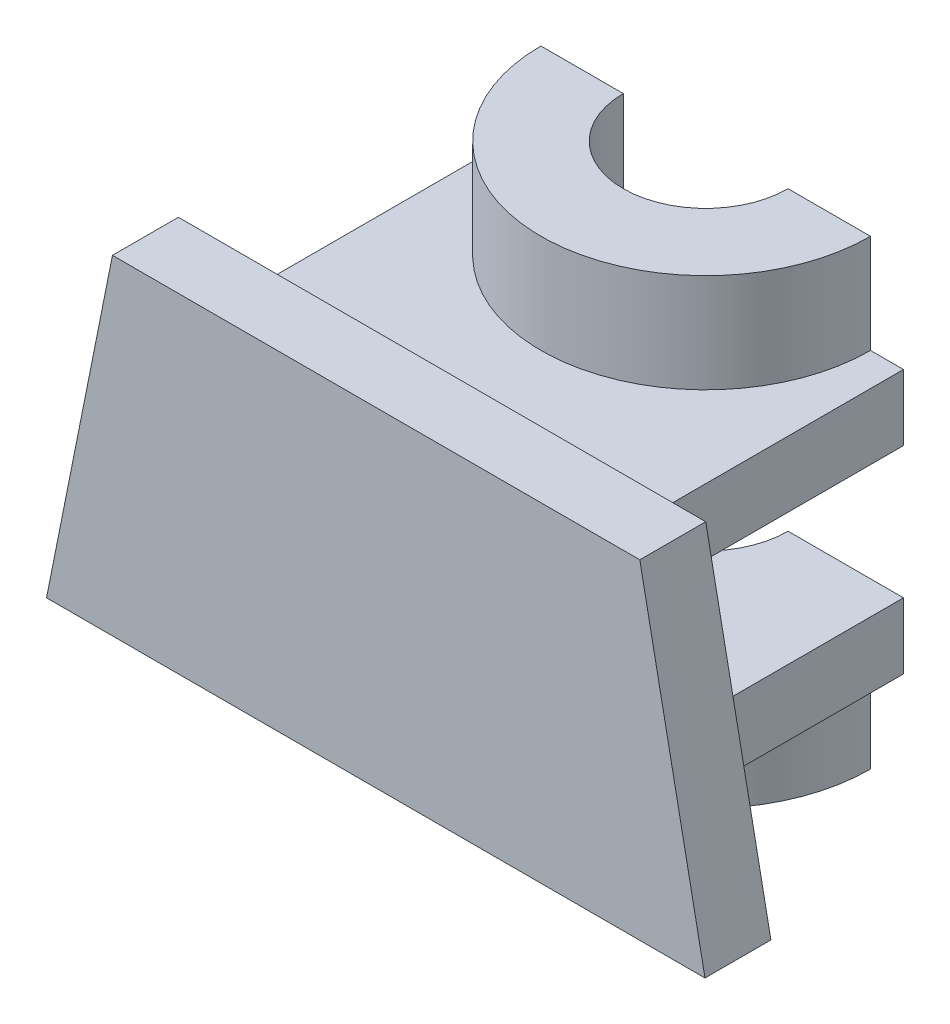
ISO-10303-21;
HEADER;
FILE_DESCRIPTION(('STEP AP214'),'2;1');
FILE_NAME('part.step','',(''),(''),'','','');
FILE_SCHEMA(('AUTOMOTIVE_DESIGN { 1 0 10303 214 1 1 1 1 }'));
ENDSEC;
DATA;
#1=APPLICATION_CONTEXT('core data for automotive mechanical design processes');
#2=APPLICATION_PROTOCOL_DEFINITION('international standard','automotive_design',2000,#1);
#3=PRODUCT_CONTEXT('',#1,'mechanical');
#4=PRODUCT('Part','Part','',(#3));
#5=PRODUCT_RELATED_PRODUCT_CATEGORY('part','',(#4));
#6=PRODUCT_DEFINITION_FORMATION('','',#4);
#7=PRODUCT_DEFINITION_CONTEXT('part definition',#1,'design');
#8=PRODUCT_DEFINITION('design','',#6,#7);
#9=PRODUCT_DEFINITION_SHAPE('','',#8);
#10=(LENGTH_UNIT() NAMED_UNIT(*) SI_UNIT(.MILLI.,.METRE.));
#11=(NAMED_UNIT(*) PLANE_ANGLE_UNIT() SI_UNIT($,.RADIAN.));
#12=(NAMED_UNIT(*) SI_UNIT($,.STERADIAN.) SOLID_ANGLE_UNIT());
#13=UNCERTAINTY_MEASURE_WITH_UNIT(LENGTH_MEASURE(1.E-05),#10,'distance_accuracy_value','');
#14=(GEOMETRIC_REPRESENTATION_CONTEXT(3) GLOBAL_UNCERTAINTY_ASSIGNED_CONTEXT((#13)) GLOBAL_UNIT_ASSIGNED_CONTEXT((#10,
#11,#12)) REPRESENTATION_CONTEXT('',''));
#15=CARTESIAN_POINT('',(0.,0.,0.));
#16=DIRECTION('',(0.,0.,1.));
#17=DIRECTION('',(1.,0.,0.));
#18=AXIS2_PLACEMENT_3D('',#15,#16,#17);
#19=CARTESIAN_POINT('',(0.,45.,0.));
#20=DIRECTION('',(0.,-1.,0.));
#21=DIRECTION('',(0.,0.,-1.));
#22=AXIS2_PLACEMENT_3D('',#19,#20,#21);
#23=PLANE('',#22);
#24=CARTESIAN_POINT('',(50.,45.,-40.));
#25=DIRECTION('',(0.,1.,0.));
#26=DIRECTION('',(0.,0.,1.));
#27=AXIS2_PLACEMENT_3D('',#24,#25,#26);
#28=CIRCLE('',#27,25.);
#29=CARTESIAN_POINT('',(25.,45.,-40.));
#30=VERTEX_POINT('',#29);
#31=CARTESIAN_POINT('',(75.,45.,-40.));
#32=VERTEX_POINT('',#31);
#33=EDGE_CURVE('E293',#30,#32,#28,.T.);
#34=ORIENTED_EDGE('',*,*,#33,.F.);
#35=DIRECTION('',(-1.,0.,0.));
#36=VECTOR('',#35,1.);
#37=CARTESIAN_POINT('',(20.,45.,-40.));
#38=LINE('',#37,#36);
#39=CARTESIAN_POINT('',(20.,45.,-40.));
#40=VERTEX_POINT('',#39);
#41=EDGE_CURVE('E221',#30,#40,#38,.T.);
#42=ORIENTED_EDGE('',*,*,#41,.T.);
#43=DIRECTION('',(0.,0.,1.));
#44=VECTOR('',#43,1.);
#45=CARTESIAN_POINT('',(20.,45.,0.));
#46=LINE('',#45,#44);
#47=CARTESIAN_POINT('',(20.,45.,0.));
#48=VERTEX_POINT('',#47);
#49=EDGE_CURVE('E216',#40,#48,#46,.T.);
#50=ORIENTED_EDGE('',*,*,#49,.T.);
#51=DIRECTION('',(1.,0.,0.));
#52=VECTOR('',#51,1.);
#53=CARTESIAN_POINT('',(50.,45.,0.));
#54=LINE('',#53,#52);
#55=CARTESIAN_POINT('',(80.,45.,0.));
#56=VERTEX_POINT('',#55);
#57=EDGE_CURVE('E213',#48,#56,#54,.T.);
#58=ORIENTED_EDGE('',*,*,#57,.T.);
#59=DIRECTION('',(0.,0.,-1.));
#60=VECTOR('',#59,1.);
#61=CARTESIAN_POINT('',(80.,45.,-40.));
#62=LINE('',#61,#60);
#63=CARTESIAN_POINT('',(80.,45.,-40.));
#64=VERTEX_POINT('',#63);
#65=EDGE_CURVE('E228',#56,#64,#62,.T.);
#66=ORIENTED_EDGE('',*,*,#65,.T.);
#67=EDGE_CURVE('E225',#64,#32,#38,.T.);
#68=ORIENTED_EDGE('',*,*,#67,.T.);
#69=EDGE_LOOP('',(#34,#42,#50,#58,#66,#68));
#70=FACE_BOUND('',#69,.T.);
#71=ADVANCED_FACE('F39',(#70),#23,.F.);
#72=CARTESIAN_POINT('',(20.,35.,-40.));
#73=DIRECTION('',(0.,0.,-1.));
#74=DIRECTION('',(-1.,0.,0.));
#75=AXIS2_PLACEMENT_3D('',#72,#73,#74);
#76=PLANE('',#75);
#77=DIRECTION('',(0.,1.,0.));
#78=VECTOR('',#77,1.);
#79=CARTESIAN_POINT('',(37.5,0.,-40.));
#80=LINE('',#79,#78);
#81=CARTESIAN_POINT('',(37.5,35.,-40.));
#82=VERTEX_POINT('',#81);
#83=CARTESIAN_POINT('',(37.5,60.,-40.));
#84=VERTEX_POINT('',#83);
#85=EDGE_CURVE('E264',#82,#84,#80,.T.);
#86=ORIENTED_EDGE('',*,*,#85,.F.);
#87=DIRECTION('',(-1.,0.,0.));
#88=VECTOR('',#87,1.);
#89=CARTESIAN_POINT('',(20.,35.,-40.));
#90=LINE('',#89,#88);
#91=CARTESIAN_POINT('',(20.,35.,-40.));
#92=VERTEX_POINT('',#91);
#93=EDGE_CURVE('E232',#82,#92,#90,.T.);
#94=ORIENTED_EDGE('',*,*,#93,.T.);
#95=DIRECTION('',(0.,1.,0.));
#96=VECTOR('',#95,1.);
#97=CARTESIAN_POINT('',(20.,35.,-40.));
#98=LINE('',#97,#96);
#99=EDGE_CURVE('E208',#92,#40,#98,.T.);
#100=ORIENTED_EDGE('',*,*,#99,.T.);
#101=ORIENTED_EDGE('',*,*,#41,.F.);
#102=DIRECTION('',(0.,-1.,0.));
#103=VECTOR('',#102,1.);
#104=CARTESIAN_POINT('',(25.,60.,-40.));
#105=LINE('',#104,#103);
#106=CARTESIAN_POINT('',(25.,60.,-40.));
#107=VERTEX_POINT('',#106);
#108=EDGE_CURVE('E288',#107,#30,#105,.T.);
#109=ORIENTED_EDGE('',*,*,#108,.F.);
#110=DIRECTION('',(-1.,0.,0.));
#111=VECTOR('',#110,1.);
#112=CARTESIAN_POINT('',(25.,60.,-40.));
#113=LINE('',#112,#111);
#114=EDGE_CURVE('E286',#84,#107,#113,.T.);
#115=ORIENTED_EDGE('',*,*,#114,.F.);
#116=EDGE_LOOP('',(#86,#94,#100,#101,#109,#115));
#117=FACE_BOUND('',#116,.T.);
#118=ADVANCED_FACE('F345',(#117),#76,.T.);
#119=CARTESIAN_POINT('',(20.,15.,-40.));
#120=DIRECTION('',(0.,0.,1.));
#121=DIRECTION('',(1.,0.,0.));
#122=AXIS2_PLACEMENT_3D('',#119,#120,#121);
#123=PLANE('',#122);
#124=DIRECTION('',(-1.,0.,0.));
#125=VECTOR('',#124,1.);
#126=CARTESIAN_POINT('',(20.,5.,-40.));
#127=LINE('',#126,#125);
#128=CARTESIAN_POINT('',(80.,5.,-40.));
#129=VERTEX_POINT('',#128);
#130=CARTESIAN_POINT('',(75.,5.,-40.));
#131=VERTEX_POINT('',#130);
#132=EDGE_CURVE('E251',#129,#131,#127,.T.);
#133=ORIENTED_EDGE('',*,*,#132,.T.);
#134=DIRECTION('',(0.,1.,0.));
#135=VECTOR('',#134,1.);
#136=CARTESIAN_POINT('',(75.,-9.99999999999999,-40.));
#137=LINE('',#136,#135);
#138=CARTESIAN_POINT('',(75.,-9.99999999999999,-40.));
#139=VERTEX_POINT('',#138);
#140=EDGE_CURVE('E310',#139,#131,#137,.T.);
#141=ORIENTED_EDGE('',*,*,#140,.F.);
#142=DIRECTION('',(-1.,0.,0.));
#143=VECTOR('',#142,1.);
#144=CARTESIAN_POINT('',(62.5,-9.99999999999999,-40.));
#145=LINE('',#144,#143);
#146=CARTESIAN_POINT('',(62.5,-9.99999999999999,-40.));
#147=VERTEX_POINT('',#146);
#148=EDGE_CURVE('E309',#139,#147,#145,.T.);
#149=ORIENTED_EDGE('',*,*,#148,.T.);
#150=DIRECTION('',(0.,1.,0.));
#151=VECTOR('',#150,1.);
#152=CARTESIAN_POINT('',(62.5,0.,-40.));
#153=LINE('',#152,#151);
#154=CARTESIAN_POINT('',(62.5,15.,-40.));
#155=VERTEX_POINT('',#154);
#156=EDGE_CURVE('E282',#147,#155,#153,.T.);
#157=ORIENTED_EDGE('',*,*,#156,.T.);
#158=DIRECTION('',(-1.,0.,0.));
#159=VECTOR('',#158,1.);
#160=CARTESIAN_POINT('',(20.,15.,-40.));
#161=LINE('',#160,#159);
#162=CARTESIAN_POINT('',(80.,15.,-40.));
#163=VERTEX_POINT('',#162);
#164=EDGE_CURVE('E263',#163,#155,#161,.T.);
#165=ORIENTED_EDGE('',*,*,#164,.F.);
#166=DIRECTION('',(0.,-1.,0.));
#167=VECTOR('',#166,1.);
#168=CARTESIAN_POINT('',(80.,15.,-40.));
#169=LINE('',#168,#167);
#170=EDGE_CURVE('E246',#163,#129,#169,.T.);
#171=ORIENTED_EDGE('',*,*,#170,.T.);
#172=EDGE_LOOP('',(#133,#141,#149,#157,#165,#171));
#173=FACE_BOUND('',#172,.T.);
#174=ADVANCED_FACE('F346',(#173),#123,.F.);
#175=CARTESIAN_POINT('',(0.,0.,10.));
#176=DIRECTION('',(0.,1.,0.));
#177=DIRECTION('',(0.,0.,1.));
#178=AXIS2_PLACEMENT_3D('',#175,#176,#177);
#179=PLANE('',#178);
#180=DIRECTION('',(1.,0.,0.));
#181=VECTOR('',#180,1.);
#182=CARTESIAN_POINT('',(0.,0.,0.));
#183=LINE('',#182,#181);
#184=CARTESIAN_POINT('',(0.,0.,0.));
#185=VERTEX_POINT('',#184);
#186=CARTESIAN_POINT('',(99.8906286080262,0.,0.));
#187=VERTEX_POINT('',#186);
#188=EDGE_CURVE('E195',#185,#187,#183,.T.);
#189=ORIENTED_EDGE('',*,*,#188,.T.);
#190=DIRECTION('',(0.,0.,1.));
#191=VECTOR('',#190,1.);
#192=CARTESIAN_POINT('',(99.8906286080262,0.,10.));
#193=LINE('',#192,#191);
#194=CARTESIAN_POINT('',(99.8906286080262,0.,10.));
#195=VERTEX_POINT('',#194);
#196=EDGE_CURVE('E53',#187,#195,#193,.T.);
#197=ORIENTED_EDGE('',*,*,#196,.T.);
#198=DIRECTION('',(1.,0.,0.));
#199=VECTOR('',#198,1.);
#200=CARTESIAN_POINT('',(0.,0.,10.));
#201=LINE('',#200,#199);
#202=CARTESIAN_POINT('',(0.,0.,10.));
#203=VERTEX_POINT('',#202);
#204=EDGE_CURVE('E192',#203,#195,#201,.T.);
#205=ORIENTED_EDGE('',*,*,#204,.F.);
#206=DIRECTION('',(0.,0.,-1.));
#207=VECTOR('',#206,1.);
#208=CARTESIAN_POINT('',(0.,0.,10.));
#209=LINE('',#208,#207);
#210=EDGE_CURVE('E50',#203,#185,#209,.T.);
#211=ORIENTED_EDGE('',*,*,#210,.T.);
#212=EDGE_LOOP('',(#189,#197,#205,#211));
#213=FACE_BOUND('',#212,.T.);
#214=ADVANCED_FACE('F41',(#213),#179,.F.);
#215=CARTESIAN_POINT('',(100.,50.,10.));
#216=DIRECTION('',(0.,-1.,0.));
#217=DIRECTION('',(0.,0.,-1.));
#218=AXIS2_PLACEMENT_3D('',#215,#216,#217);
#219=PLANE('',#218);
#220=DIRECTION('',(-1.,0.,0.));
#221=VECTOR('',#220,1.);
#222=CARTESIAN_POINT('',(100.,50.,10.));
#223=LINE('',#222,#221);
#224=CARTESIAN_POINT('',(90.,50.,10.));
#225=VERTEX_POINT('',#224);
#226=CARTESIAN_POINT('',(9.99999999999999,50.,10.));
#227=VERTEX_POINT('',#226);
#228=EDGE_CURVE('E187',#225,#227,#223,.T.);
#229=ORIENTED_EDGE('',*,*,#228,.F.);
#230=DIRECTION('',(0.,0.,-1.));
#231=VECTOR('',#230,1.);
#232=CARTESIAN_POINT('',(90.,50.,15.));
#233=LINE('',#232,#231);
#234=CARTESIAN_POINT('',(90.,50.,0.));
#235=VERTEX_POINT('',#234);
#236=EDGE_CURVE('E172',#225,#235,#233,.T.);
#237=ORIENTED_EDGE('',*,*,#236,.T.);
#238=DIRECTION('',(-1.,0.,0.));
#239=VECTOR('',#238,1.);
#240=CARTESIAN_POINT('',(100.,50.,0.));
#241=LINE('',#240,#239);
#242=CARTESIAN_POINT('',(9.99999999999999,50.,0.));
#243=VERTEX_POINT('',#242);
#244=EDGE_CURVE('E183',#235,#243,#241,.T.);
#245=ORIENTED_EDGE('',*,*,#244,.T.);
#246=DIRECTION('',(0.,0.,-1.));
#247=VECTOR('',#246,1.);
#248=CARTESIAN_POINT('',(9.99999999999999,50.,15.));
#249=LINE('',#248,#247);
#250=EDGE_CURVE('E62',#227,#243,#249,.T.);
#251=ORIENTED_EDGE('',*,*,#250,.F.);
#252=EDGE_LOOP('',(#229,#237,#245,#251));
#253=FACE_BOUND('',#252,.T.);
#254=ADVANCED_FACE('F182',(#253),#219,.F.);
#255=CARTESIAN_POINT('',(0.,0.,10.));
#256=DIRECTION('',(0.,0.,1.));
#257=DIRECTION('',(1.,0.,0.));
#258=AXIS2_PLACEMENT_3D('',#255,#256,#257);
#259=PLANE('',#258);
#260=DIRECTION('',(0.194052386180956,-0.980991167859057,0.));
#261=VECTOR('',#260,1.);
#262=CARTESIAN_POINT('',(96.1291142748476,19.0155473542205,10.));
#263=LINE('',#262,#261);
#264=EDGE_CURVE('E323',#225,#195,#263,.T.);
#265=ORIENTED_EDGE('',*,*,#264,.F.);
#266=ORIENTED_EDGE('',*,*,#228,.T.);
#267=DIRECTION('',(0.196116135138184,0.98058067569092,0.));
#268=VECTOR('',#267,1.);
#269=CARTESIAN_POINT('',(0.,0.,10.));
#270=LINE('',#269,#268);
#271=EDGE_CURVE('E190',#203,#227,#270,.T.);
#272=ORIENTED_EDGE('',*,*,#271,.F.);
#273=ORIENTED_EDGE('',*,*,#204,.T.);
#274=EDGE_LOOP('',(#265,#266,#272,#273));
#275=FACE_BOUND('',#274,.T.);
#276=ADVANCED_FACE('F328',(#275),#259,.T.);
#277=CARTESIAN_POINT('',(0.,0.,0.));
#278=DIRECTION('',(0.,0.,1.));
#279=DIRECTION('',(1.,0.,0.));
#280=AXIS2_PLACEMENT_3D('',#277,#278,#279);
#281=PLANE('',#280);
#282=DIRECTION('',(0.,-1.,0.));
#283=VECTOR('',#282,1.);
#284=CARTESIAN_POINT('',(80.,15.,0.));
#285=LINE('',#284,#283);
#286=CARTESIAN_POINT('',(80.,15.,0.));
#287=VERTEX_POINT('',#286);
#288=CARTESIAN_POINT('',(80.,5.,0.));
#289=VERTEX_POINT('',#288);
#290=EDGE_CURVE('E230',#287,#289,#285,.T.);
#291=ORIENTED_EDGE('',*,*,#290,.F.);
#292=DIRECTION('',(1.,0.,0.));
#293=VECTOR('',#292,1.);
#294=CARTESIAN_POINT('',(80.,15.,0.));
#295=LINE('',#294,#293);
#296=CARTESIAN_POINT('',(20.,15.,0.));
#297=VERTEX_POINT('',#296);
#298=EDGE_CURVE('E254',#297,#287,#295,.T.);
#299=ORIENTED_EDGE('',*,*,#298,.F.);
#300=DIRECTION('',(0.,-1.,0.));
#301=VECTOR('',#300,1.);
#302=CARTESIAN_POINT('',(20.,15.,0.));
#303=LINE('',#302,#301);
#304=CARTESIAN_POINT('',(20.,5.,0.));
#305=VERTEX_POINT('',#304);
#306=EDGE_CURVE('E239',#297,#305,#303,.T.);
#307=ORIENTED_EDGE('',*,*,#306,.T.);
#308=DIRECTION('',(1.,0.,0.));
#309=VECTOR('',#308,1.);
#310=CARTESIAN_POINT('',(50.,5.,0.));
#311=LINE('',#310,#309);
#312=EDGE_CURVE('E262',#305,#289,#311,.T.);
#313=ORIENTED_EDGE('',*,*,#312,.T.);
#314=EDGE_LOOP('',(#291,#299,#307,#313));
#315=FACE_BOUND('',#314,.T.);
#316=DIRECTION('',(0.,1.,0.));
#317=VECTOR('',#316,1.);
#318=CARTESIAN_POINT('',(20.,35.,0.));
#319=LINE('',#318,#317);
#320=CARTESIAN_POINT('',(20.,35.,0.));
#321=VERTEX_POINT('',#320);
#322=EDGE_CURVE('E197',#321,#48,#319,.T.);
#323=ORIENTED_EDGE('',*,*,#322,.F.);
#324=DIRECTION('',(1.,0.,0.));
#325=VECTOR('',#324,1.);
#326=CARTESIAN_POINT('',(80.,35.,0.));
#327=LINE('',#326,#325);
#328=CARTESIAN_POINT('',(80.,35.,0.));
#329=VERTEX_POINT('',#328);
#330=EDGE_CURVE('E219',#321,#329,#327,.T.);
#331=ORIENTED_EDGE('',*,*,#330,.T.);
#332=DIRECTION('',(0.,1.,0.));
#333=VECTOR('',#332,1.);
#334=CARTESIAN_POINT('',(80.,35.,0.));
#335=LINE('',#334,#333);
#336=EDGE_CURVE('E201',#329,#56,#335,.T.);
#337=ORIENTED_EDGE('',*,*,#336,.T.);
#338=ORIENTED_EDGE('',*,*,#57,.F.);
#339=EDGE_LOOP('',(#323,#331,#337,#338));
#340=FACE_BOUND('',#339,.T.);
#341=ORIENTED_EDGE('',*,*,#244,.F.);
#342=DIRECTION('',(0.194052386180956,-0.980991167859057,0.));
#343=VECTOR('',#342,1.);
#344=CARTESIAN_POINT('',(96.1291142748476,19.0155473542205,0.));
#345=LINE('',#344,#343);
#346=EDGE_CURVE('E11',#235,#187,#345,.T.);
#347=ORIENTED_EDGE('',*,*,#346,.T.);
#348=ORIENTED_EDGE('',*,*,#188,.F.);
#349=DIRECTION('',(-0.196116135138184,-0.98058067569092,0.));
#350=VECTOR('',#349,1.);
#351=CARTESIAN_POINT('',(9.99999999999999,50.,0.));
#352=LINE('',#351,#350);
#353=EDGE_CURVE('E188',#243,#185,#352,.T.);
#354=ORIENTED_EDGE('',*,*,#353,.F.);
#355=EDGE_LOOP('',(#341,#347,#348,#354));
#356=FACE_BOUND('',#355,.T.);
#357=ADVANCED_FACE('F186',(#315,#340,#356),#281,.F.);
#358=CARTESIAN_POINT('',(20.,35.,0.));
#359=DIRECTION('',(-1.,0.,0.));
#360=DIRECTION('',(0.,0.,1.));
#361=AXIS2_PLACEMENT_3D('',#358,#359,#360);
#362=PLANE('',#361);
#363=ORIENTED_EDGE('',*,*,#49,.F.);
#364=ORIENTED_EDGE('',*,*,#99,.F.);
#365=DIRECTION('',(0.,0.,1.));
#366=VECTOR('',#365,1.);
#367=CARTESIAN_POINT('',(20.,35.,0.));
#368=LINE('',#367,#366);
#369=EDGE_CURVE('E206',#92,#321,#368,.T.);
#370=ORIENTED_EDGE('',*,*,#369,.T.);
#371=ORIENTED_EDGE('',*,*,#322,.T.);
#372=EDGE_LOOP('',(#363,#364,#370,#371));
#373=FACE_BOUND('',#372,.T.);
#374=ADVANCED_FACE('F340',(#373),#362,.T.);
#375=DIRECTION('',(0.,1.,0.));
#376=VECTOR('',#375,1.);
#377=CARTESIAN_POINT('',(62.5,0.,-40.));
#378=LINE('',#377,#376);
#379=CARTESIAN_POINT('',(62.5,60.,-40.));
#380=VERTEX_POINT('',#379);
#381=CARTESIAN_POINT('',(62.5,35.,-40.));
#382=VERTEX_POINT('',#381);
#383=EDGE_CURVE('E273',#380,#382,#378,.F.);
#384=ORIENTED_EDGE('',*,*,#383,.F.);
#385=DIRECTION('',(-1.,0.,0.));
#386=VECTOR('',#385,1.);
#387=CARTESIAN_POINT('',(62.5,60.,-40.));
#388=LINE('',#387,#386);
#389=CARTESIAN_POINT('',(75.,60.,-40.));
#390=VERTEX_POINT('',#389);
#391=EDGE_CURVE('E297',#390,#380,#388,.T.);
#392=ORIENTED_EDGE('',*,*,#391,.F.);
#393=DIRECTION('',(0.,-1.,0.));
#394=VECTOR('',#393,1.);
#395=CARTESIAN_POINT('',(75.,60.,-40.));
#396=LINE('',#395,#394);
#397=EDGE_CURVE('E287',#390,#32,#396,.T.);
#398=ORIENTED_EDGE('',*,*,#397,.T.);
#399=ORIENTED_EDGE('',*,*,#67,.F.);
#400=DIRECTION('',(0.,1.,0.));
#401=VECTOR('',#400,1.);
#402=CARTESIAN_POINT('',(80.,35.,-40.));
#403=LINE('',#402,#401);
#404=CARTESIAN_POINT('',(80.,35.,-40.));
#405=VERTEX_POINT('',#404);
#406=EDGE_CURVE('E210',#405,#64,#403,.T.);
#407=ORIENTED_EDGE('',*,*,#406,.F.);
#408=EDGE_CURVE('E235',#405,#382,#90,.T.);
#409=ORIENTED_EDGE('',*,*,#408,.T.);
#410=EDGE_LOOP('',(#384,#392,#398,#399,#407,#409));
#411=FACE_BOUND('',#410,.T.);
#412=ADVANCED_FACE('F355',(#411),#76,.T.);
#413=CARTESIAN_POINT('',(80.,35.,-40.));
#414=DIRECTION('',(1.,0.,0.));
#415=DIRECTION('',(0.,0.,-1.));
#416=AXIS2_PLACEMENT_3D('',#413,#414,#415);
#417=PLANE('',#416);
#418=ORIENTED_EDGE('',*,*,#65,.F.);
#419=ORIENTED_EDGE('',*,*,#336,.F.);
#420=DIRECTION('',(0.,0.,-1.));
#421=VECTOR('',#420,1.);
#422=CARTESIAN_POINT('',(80.,35.,-40.));
#423=LINE('',#422,#421);
#424=EDGE_CURVE('E236',#329,#405,#423,.T.);
#425=ORIENTED_EDGE('',*,*,#424,.T.);
#426=ORIENTED_EDGE('',*,*,#406,.T.);
#427=EDGE_LOOP('',(#418,#419,#425,#426));
#428=FACE_BOUND('',#427,.T.);
#429=ADVANCED_FACE('F363',(#428),#417,.T.);
#430=CARTESIAN_POINT('',(0.,35.,0.));
#431=DIRECTION('',(0.,-1.,0.));
#432=DIRECTION('',(0.,0.,-1.));
#433=AXIS2_PLACEMENT_3D('',#430,#431,#432);
#434=PLANE('',#433);
#435=CARTESIAN_POINT('',(50.,35.,-40.));
#436=DIRECTION('',(0.,-1.,0.));
#437=DIRECTION('',(0.,0.,-1.));
#438=AXIS2_PLACEMENT_3D('',#435,#436,#437);
#439=CIRCLE('',#438,12.5);
#440=EDGE_CURVE('E280',#382,#82,#439,.T.);
#441=ORIENTED_EDGE('',*,*,#440,.F.);
#442=ORIENTED_EDGE('',*,*,#408,.F.);
#443=ORIENTED_EDGE('',*,*,#424,.F.);
#444=ORIENTED_EDGE('',*,*,#330,.F.);
#445=ORIENTED_EDGE('',*,*,#369,.F.);
#446=ORIENTED_EDGE('',*,*,#93,.F.);
#447=EDGE_LOOP('',(#441,#442,#443,#444,#445,#446));
#448=FACE_BOUND('',#447,.T.);
#449=ADVANCED_FACE('F358',(#448),#434,.T.);
#450=CARTESIAN_POINT('',(80.,15.,-40.));
#451=DIRECTION('',(-1.,0.,0.));
#452=DIRECTION('',(0.,0.,1.));
#453=AXIS2_PLACEMENT_3D('',#450,#451,#452);
#454=PLANE('',#453);
#455=DIRECTION('',(0.,0.,-1.));
#456=VECTOR('',#455,1.);
#457=CARTESIAN_POINT('',(80.,5.,-40.));
#458=LINE('',#457,#456);
#459=EDGE_CURVE('E252',#289,#129,#458,.T.);
#460=ORIENTED_EDGE('',*,*,#459,.T.);
#461=ORIENTED_EDGE('',*,*,#170,.F.);
#462=DIRECTION('',(0.,0.,-1.));
#463=VECTOR('',#462,1.);
#464=CARTESIAN_POINT('',(80.,15.,-40.));
#465=LINE('',#464,#463);
#466=EDGE_CURVE('E243',#287,#163,#465,.T.);
#467=ORIENTED_EDGE('',*,*,#466,.F.);
#468=ORIENTED_EDGE('',*,*,#290,.T.);
#469=EDGE_LOOP('',(#460,#461,#467,#468));
#470=FACE_BOUND('',#469,.T.);
#471=ADVANCED_FACE('F367',(#470),#454,.F.);
#472=CARTESIAN_POINT('',(37.5,15.,-40.));
#473=VERTEX_POINT('',#472);
#474=CARTESIAN_POINT('',(20.,15.,-40.));
#475=VERTEX_POINT('',#474);
#476=EDGE_CURVE('E268',#473,#475,#161,.T.);
#477=ORIENTED_EDGE('',*,*,#476,.F.);
#478=DIRECTION('',(0.,1.,0.));
#479=VECTOR('',#478,1.);
#480=CARTESIAN_POINT('',(37.5,0.,-40.));
#481=LINE('',#480,#479);
#482=CARTESIAN_POINT('',(37.5,-9.99999999999999,-40.));
#483=VERTEX_POINT('',#482);
#484=EDGE_CURVE('E281',#473,#483,#481,.F.);
#485=ORIENTED_EDGE('',*,*,#484,.T.);
#486=DIRECTION('',(-1.,0.,0.));
#487=VECTOR('',#486,1.);
#488=CARTESIAN_POINT('',(25.,-9.99999999999999,-40.));
#489=LINE('',#488,#487);
#490=CARTESIAN_POINT('',(25.,-9.99999999999999,-40.));
#491=VERTEX_POINT('',#490);
#492=EDGE_CURVE('E316',#483,#491,#489,.T.);
#493=ORIENTED_EDGE('',*,*,#492,.T.);
#494=DIRECTION('',(0.,1.,0.));
#495=VECTOR('',#494,1.);
#496=CARTESIAN_POINT('',(25.,-9.99999999999999,-40.));
#497=LINE('',#496,#495);
#498=CARTESIAN_POINT('',(25.,5.,-40.));
#499=VERTEX_POINT('',#498);
#500=EDGE_CURVE('E294',#491,#499,#497,.T.);
#501=ORIENTED_EDGE('',*,*,#500,.T.);
#502=CARTESIAN_POINT('',(20.,5.,-40.));
#503=VERTEX_POINT('',#502);
#504=EDGE_CURVE('E260',#499,#503,#127,.T.);
#505=ORIENTED_EDGE('',*,*,#504,.T.);
#506=DIRECTION('',(0.,-1.,0.));
#507=VECTOR('',#506,1.);
#508=CARTESIAN_POINT('',(20.,15.,-40.));
#509=LINE('',#508,#507);
#510=EDGE_CURVE('E245',#475,#503,#509,.T.);
#511=ORIENTED_EDGE('',*,*,#510,.F.);
#512=EDGE_LOOP('',(#477,#485,#493,#501,#505,#511));
#513=FACE_BOUND('',#512,.T.);
#514=ADVANCED_FACE('F421',(#513),#123,.F.);
#515=CARTESIAN_POINT('',(20.,15.,0.));
#516=DIRECTION('',(1.,0.,0.));
#517=DIRECTION('',(0.,0.,-1.));
#518=AXIS2_PLACEMENT_3D('',#515,#516,#517);
#519=PLANE('',#518);
#520=DIRECTION('',(0.,0.,1.));
#521=VECTOR('',#520,1.);
#522=CARTESIAN_POINT('',(20.,5.,0.));
#523=LINE('',#522,#521);
#524=EDGE_CURVE('E259',#503,#305,#523,.T.);
#525=ORIENTED_EDGE('',*,*,#524,.T.);
#526=ORIENTED_EDGE('',*,*,#306,.F.);
#527=DIRECTION('',(0.,0.,1.));
#528=VECTOR('',#527,1.);
#529=CARTESIAN_POINT('',(20.,15.,0.));
#530=LINE('',#529,#528);
#531=EDGE_CURVE('E269',#475,#297,#530,.T.);
#532=ORIENTED_EDGE('',*,*,#531,.F.);
#533=ORIENTED_EDGE('',*,*,#510,.T.);
#534=EDGE_LOOP('',(#525,#526,#532,#533));
#535=FACE_BOUND('',#534,.T.);
#536=ADVANCED_FACE('F420',(#535),#519,.F.);
#537=CARTESIAN_POINT('',(0.,15.,0.));
#538=DIRECTION('',(0.,1.,0.));
#539=DIRECTION('',(0.,0.,-1.));
#540=AXIS2_PLACEMENT_3D('',#537,#538,#539);
#541=PLANE('',#540);
#542=CARTESIAN_POINT('',(50.,15.,-40.));
#543=DIRECTION('',(0.,1.,0.));
#544=DIRECTION('',(0.,0.,1.));
#545=AXIS2_PLACEMENT_3D('',#542,#543,#544);
#546=CIRCLE('',#545,12.5);
#547=EDGE_CURVE('E276',#473,#155,#546,.T.);
#548=ORIENTED_EDGE('',*,*,#547,.F.);
#549=ORIENTED_EDGE('',*,*,#476,.T.);
#550=ORIENTED_EDGE('',*,*,#531,.T.);
#551=ORIENTED_EDGE('',*,*,#298,.T.);
#552=ORIENTED_EDGE('',*,*,#466,.T.);
#553=ORIENTED_EDGE('',*,*,#164,.T.);
#554=EDGE_LOOP('',(#548,#549,#550,#551,#552,#553));
#555=FACE_BOUND('',#554,.T.);
#556=ADVANCED_FACE('F413',(#555),#541,.T.);
#557=CARTESIAN_POINT('',(0.,5.,0.));
#558=DIRECTION('',(0.,1.,0.));
#559=DIRECTION('',(0.,0.,-1.));
#560=AXIS2_PLACEMENT_3D('',#557,#558,#559);
#561=PLANE('',#560);
#562=ORIENTED_EDGE('',*,*,#504,.F.);
#563=CARTESIAN_POINT('',(50.,5.,-40.));
#564=DIRECTION('',(0.,1.,0.));
#565=DIRECTION('',(0.,0.,1.));
#566=AXIS2_PLACEMENT_3D('',#563,#564,#565);
#567=CIRCLE('',#566,25.);
#568=EDGE_CURVE('E311',#499,#131,#567,.T.);
#569=ORIENTED_EDGE('',*,*,#568,.T.);
#570=ORIENTED_EDGE('',*,*,#132,.F.);
#571=ORIENTED_EDGE('',*,*,#459,.F.);
#572=ORIENTED_EDGE('',*,*,#312,.F.);
#573=ORIENTED_EDGE('',*,*,#524,.F.);
#574=EDGE_LOOP('',(#562,#569,#570,#571,#572,#573));
#575=FACE_BOUND('',#574,.T.);
#576=ADVANCED_FACE('F414',(#575),#561,.F.);
#577=CARTESIAN_POINT('',(50.,0.,-40.));
#578=DIRECTION('',(0.,1.,0.));
#579=DIRECTION('',(0.,0.,1.));
#580=AXIS2_PLACEMENT_3D('',#577,#578,#579);
#581=CYLINDRICAL_SURFACE('',#580,12.5);
#582=ORIENTED_EDGE('',*,*,#547,.T.);
#583=ORIENTED_EDGE('',*,*,#156,.F.);
#584=CARTESIAN_POINT('',(50.,-9.99999999999999,-40.));
#585=DIRECTION('',(0.,-1.,0.));
#586=DIRECTION('',(0.,0.,1.));
#587=AXIS2_PLACEMENT_3D('',#584,#585,#586);
#588=CIRCLE('',#587,12.5);
#589=EDGE_CURVE('E317',#147,#483,#588,.T.);
#590=ORIENTED_EDGE('',*,*,#589,.T.);
#591=ORIENTED_EDGE('',*,*,#484,.F.);
#592=EDGE_LOOP('',(#582,#583,#590,#591));
#593=FACE_BOUND('',#592,.T.);
#594=ADVANCED_FACE('F408',(#593),#581,.F.);
#595=ORIENTED_EDGE('',*,*,#85,.T.);
#596=CARTESIAN_POINT('',(50.,60.,-40.));
#597=DIRECTION('',(0.,-1.,0.));
#598=DIRECTION('',(0.,0.,1.));
#599=AXIS2_PLACEMENT_3D('',#596,#597,#598);
#600=CIRCLE('',#599,12.5);
#601=EDGE_CURVE('E300',#380,#84,#600,.T.);
#602=ORIENTED_EDGE('',*,*,#601,.F.);
#603=ORIENTED_EDGE('',*,*,#383,.T.);
#604=ORIENTED_EDGE('',*,*,#440,.T.);
#605=EDGE_LOOP('',(#595,#602,#603,#604));
#606=FACE_BOUND('',#605,.T.);
#607=ADVANCED_FACE('F394',(#606),#581,.F.);
#608=CARTESIAN_POINT('',(50.,60.,-40.));
#609=DIRECTION('',(0.,-1.,0.));
#610=DIRECTION('',(0.,0.,-1.));
#611=AXIS2_PLACEMENT_3D('',#608,#609,#610);
#612=CYLINDRICAL_SURFACE('',#611,25.);
#613=ORIENTED_EDGE('',*,*,#33,.T.);
#614=ORIENTED_EDGE('',*,*,#397,.F.);
#615=CARTESIAN_POINT('',(50.,60.,-40.));
#616=DIRECTION('',(0.,1.,0.));
#617=DIRECTION('',(0.,0.,1.));
#618=AXIS2_PLACEMENT_3D('',#615,#616,#617);
#619=CIRCLE('',#618,25.);
#620=EDGE_CURVE('E295',#107,#390,#619,.T.);
#621=ORIENTED_EDGE('',*,*,#620,.F.);
#622=ORIENTED_EDGE('',*,*,#108,.T.);
#623=EDGE_LOOP('',(#613,#614,#621,#622));
#624=FACE_BOUND('',#623,.T.);
#625=ADVANCED_FACE('F387',(#624),#612,.T.);
#626=CARTESIAN_POINT('',(50.,60.,-40.));
#627=DIRECTION('',(0.,1.,0.));
#628=DIRECTION('',(0.,0.,1.));
#629=AXIS2_PLACEMENT_3D('',#626,#627,#628);
#630=PLANE('',#629);
#631=ORIENTED_EDGE('',*,*,#620,.T.);
#632=ORIENTED_EDGE('',*,*,#391,.T.);
#633=ORIENTED_EDGE('',*,*,#601,.T.);
#634=ORIENTED_EDGE('',*,*,#114,.T.);
#635=EDGE_LOOP('',(#631,#632,#633,#634));
#636=FACE_BOUND('',#635,.T.);
#637=ADVANCED_FACE('F393',(#636),#630,.T.);
#638=CARTESIAN_POINT('',(50.,-9.99999999999999,-40.));
#639=DIRECTION('',(0.,1.,0.));
#640=DIRECTION('',(0.,0.,1.));
#641=AXIS2_PLACEMENT_3D('',#638,#639,#640);
#642=CYLINDRICAL_SURFACE('',#641,25.);
#643=ORIENTED_EDGE('',*,*,#568,.F.);
#644=ORIENTED_EDGE('',*,*,#500,.F.);
#645=CARTESIAN_POINT('',(50.,-9.99999999999999,-40.));
#646=DIRECTION('',(0.,1.,0.));
#647=DIRECTION('',(0.,0.,1.));
#648=AXIS2_PLACEMENT_3D('',#645,#646,#647);
#649=CIRCLE('',#648,25.);
#650=EDGE_CURVE('E312',#491,#139,#649,.T.);
#651=ORIENTED_EDGE('',*,*,#650,.T.);
#652=ORIENTED_EDGE('',*,*,#140,.T.);
#653=EDGE_LOOP('',(#643,#644,#651,#652));
#654=FACE_BOUND('',#653,.T.);
#655=ADVANCED_FACE('F400',(#654),#642,.T.);
#656=CARTESIAN_POINT('',(50.,-9.99999999999999,-40.));
#657=DIRECTION('',(0.,-1.,0.));
#658=DIRECTION('',(0.,0.,1.));
#659=AXIS2_PLACEMENT_3D('',#656,#657,#658);
#660=PLANE('',#659);
#661=ORIENTED_EDGE('',*,*,#650,.F.);
#662=ORIENTED_EDGE('',*,*,#492,.F.);
#663=ORIENTED_EDGE('',*,*,#589,.F.);
#664=ORIENTED_EDGE('',*,*,#148,.F.);
#665=EDGE_LOOP('',(#661,#662,#663,#664));
#666=FACE_BOUND('',#665,.T.);
#667=ADVANCED_FACE('F404',(#666),#660,.T.);
#668=CARTESIAN_POINT('',(9.99999999999999,50.,15.));
#669=DIRECTION('',(0.98058067569092,-0.196116135138184,0.));
#670=DIRECTION('',(0.196116135138184,0.98058067569092,0.));
#671=AXIS2_PLACEMENT_3D('',#668,#669,#670);
#672=PLANE('',#671);
#673=ORIENTED_EDGE('',*,*,#271,.T.);
#674=ORIENTED_EDGE('',*,*,#250,.T.);
#675=ORIENTED_EDGE('',*,*,#353,.T.);
#676=ORIENTED_EDGE('',*,*,#210,.F.);
#677=EDGE_LOOP('',(#673,#674,#675,#676));
#678=FACE_BOUND('',#677,.T.);
#679=ADVANCED_FACE('F326',(#678),#672,.F.);
#680=CARTESIAN_POINT('',(90.,50.,15.));
#681=DIRECTION('',(-0.980991167859057,-0.194052386180956,0.));
#682=DIRECTION('',(0.194052386180956,-0.980991167859057,0.));
#683=AXIS2_PLACEMENT_3D('',#680,#681,#682);
#684=PLANE('',#683);
#685=ORIENTED_EDGE('',*,*,#346,.F.);
#686=ORIENTED_EDGE('',*,*,#236,.F.);
#687=ORIENTED_EDGE('',*,*,#264,.T.);
#688=ORIENTED_EDGE('',*,*,#196,.F.);
#689=EDGE_LOOP('',(#685,#686,#687,#688));
#690=FACE_BOUND('',#689,.T.);
#691=ADVANCED_FACE('F173',(#690),#684,.F.);
#692=CLOSED_SHELL('',(#71,#118,#174,#214,#254,#276,#357,#374,#412,#429,#449,#471,#514,#536,#556,
#576,#594,#607,#625,#637,#655,#667,#679,#691));
#693=MANIFOLD_SOLID_BREP('B2',#692);
#694=ADVANCED_BREP_SHAPE_REPRESENTATION('',(#18,#693),#14);
#695=SHAPE_DEFINITION_REPRESENTATION(#9,#694);
ENDSEC;
END-ISO-10303-21;
